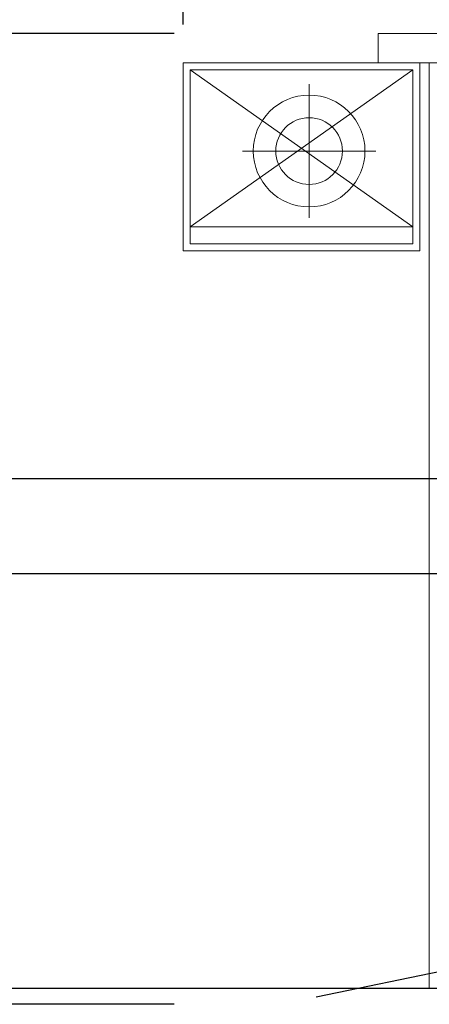
# Model space of a CAD drawing. Units: inches. Extents: x 2025 to 2528, y 1525 to 2336.
# Tile 11 of 18: x 2109 to 2138, y 2209 to 2278. Entities that reach past the tile are written whole.
import ezdxf

# ---------------------------------------------------------------- set-up
doc = ezdxf.new("R2010")
doc.units = ezdxf.units.IN
doc.layers.add('A-ANNO-DIMS', color=2, linetype='Continuous', lineweight=18)
doc.layers.add('A-FURN', color=8, linetype='Continuous', lineweight=18)
doc.styles.get("Standard").update_dxf_attribs({"font": 'arial.ttf'})
doc.dimstyles.new('Copy of ISO-25', dxfattribs={"dimtxt": 2.5, "dimasz": 2.5, "dimexe": 1.25, "dimexo": 0.625, "dimtad": 1, "dimdec": 1, "dimlunit": 4, "dimtxsty": 'Standard', "dimcen": 2.5, "dimadec": 0, "dimazin": 0, "dimtfac": 1, "dimtdec": 1, "dimtmove": 0, "dimatfit": 3, "dimfxl": 1, "dimarcsym": 0})

# ---------------------------------------------------------------- blocks, each defined once
blk = doc.blocks.new('*D6')
at = {"layer": 'A-ANNO-DIMS', "color": 0, "lineweight": -2, "transparency": 16777216}
for p, q in [((2075.013, 2282.787), (2075.013, 2237.927)), ((2255.013, 2282.787), (2255.013, 2237.927)), ((2077.513, 2239.177), (2252.513, 2239.177))]:
    blk.add_line(p, q, dxfattribs=at)
at = {"layer": 'A-ANNO-DIMS', "color": 0, "transparency": 16777216}
for points in [[(2077.513, 2239.594), (2077.513, 2238.761), (2075.013, 2239.177)], [(2252.513, 2239.594), (2252.513, 2238.761), (2255.013, 2239.177)]]:
    blk.add_solid(points, dxfattribs=at)
at = {"layer": 'Defpoints', "color": 0, "transparency": 16777216}
for p in [(2075.013, 2283.412), (2255.013, 2283.412), (2255.013, 2239.177)]:
    blk.add_point(p, dxfattribs=at)
at = {"layer": 'A-ANNO-DIMS', "color": 0, "transparency": 16777216, "insert": (2165.013, 2241.079), "char_height": 2.5, "attachment_point": 5}
blk.add_mtext("15'", dxfattribs=at)
blk = doc.blocks.new('A$C029D5C69')
for p, q in [((0.4164, 2.0693), (0.4164, 2.0066)), ((2.2315, 2.0693), (0.4164, 2.0693)), ((0, 1.606), (0, 2.0066)), ((0, 2.0066), (0.505, 2.0066)), ((0.4164, 2.0066), (2.2315, 2.0066)), ((0.505, 2.0066), (0.505, 1.606)), ((0.5252, 0.0351), (0.5252, 2.0066)), ((0.0151, 1.6211), (0.0151, 1.9915)), ((0.0151, 1.9915), (0.4899, 1.9915)), ((0.4899, 1.9915), (0.4899, 1.6211)), ((0.2689, 1.9609), (0.2689, 1.6764)), ((0.1267, 1.8186), (0.4111, 1.8186)), ((0.4899, 1.6211), (0.0151, 1.6211)), ((0.505, 1.606), (0, 1.606))]:
    blk.add_line(p, q)
at = {"ltscale": 0.005}
for p, q in [((0.4899, 1.6568), (0.0151, 1.9915)), ((0.0151, 1.6568), (0.4899, 1.9915)), ((0.0151, 1.6568), (0.4899, 1.6568))]:
    blk.add_line(p, q, dxfattribs=at)
for radius in [0.1191, 0.0711]:
    blk.add_circle((0.2689, 1.8186), radius)
blk = doc.blocks.new('*D56')
at = {"layer": 'A-ANNO-DIMS', "color": 0, "lineweight": -2, "transparency": 16777216}
for p, q in [((2120.208, 2277.944), (2120.208, 2291.728)), ((2207.933, 2277.944), (2207.933, 2291.728)), ((2122.708, 2290.478), (2205.433, 2290.478))]:
    blk.add_line(p, q, dxfattribs=at)
at = {"layer": 'A-ANNO-DIMS', "color": 0, "transparency": 16777216}
for points in [[(2122.708, 2290.895), (2122.708, 2290.061), (2120.208, 2290.478)], [(2205.433, 2290.895), (2205.433, 2290.061), (2207.933, 2290.478)]]:
    blk.add_solid(points, dxfattribs=at)
at = {"layer": 'Defpoints', "color": 0, "transparency": 16777216}
for p in [(2207.933, 2290.478), (2120.208, 2277.319), (2207.933, 2277.319)]:
    blk.add_point(p, dxfattribs=at)
at = {"layer": 'A-ANNO-DIMS', "color": 0, "transparency": 16777216, "insert": (2164.07, 2292.403), "char_height": 2.5, "attachment_point": 5}
blk.add_mtext('BED & NIGHTSTANDS 7\'-3 1/2" TYP.', dxfattribs=at)
blk = doc.blocks.new('*D57')
at = {"layer": 'A-ANNO-DIMS', "color": 0, "lineweight": -2, "transparency": 16777216}
for p, q in [((2119.583, 2277.319), (2105.799, 2277.319)), ((2107.049, 2211.264), (2107.049, 2274.819)), ((2119.583, 2208.764), (2105.799, 2208.764))]:
    blk.add_line(p, q, dxfattribs=at)
at = {"layer": 'A-ANNO-DIMS', "color": 0, "transparency": 16777216}
for points in [[(2106.632, 2274.819), (2107.466, 2274.819), (2107.049, 2277.319)], [(2106.632, 2211.264), (2107.466, 2211.264), (2107.049, 2208.764)]]:
    blk.add_solid(points, dxfattribs=at)
at = {"layer": 'Defpoints', "color": 0, "transparency": 16777216}
for p in [(2107.049, 2277.319), (2120.208, 2277.319), (2120.208, 2208.764)]:
    blk.add_point(p, dxfattribs=at)
at = {"layer": 'A-ANNO-DIMS', "color": 0, "transparency": 16777216, "insert": (2105.131, 2243.042), "char_height": 2.5, "attachment_point": 5, "rotation": 90}
blk.add_mtext('5\'-8 1/2" TYP.', dxfattribs=at)
blk = doc.blocks.new('*D78')
at = {"layer": 'A-ANNO-DIMS', "color": 0, "lineweight": -2, "transparency": 16777216}
for p, q in [((2254.388, 2245.877), (2027.213, 2245.877)), ((2028.463, 2212.377), (2028.463, 2243.377)), ((2254.388, 2209.877), (2027.213, 2209.877))]:
    blk.add_line(p, q, dxfattribs=at)
at = {"layer": 'A-ANNO-DIMS', "color": 0, "transparency": 16777216}
for points in [[(2028.046, 2243.377), (2028.88, 2243.377), (2028.463, 2245.877)], [(2028.046, 2212.377), (2028.88, 2212.377), (2028.463, 2209.877)]]:
    blk.add_solid(points, dxfattribs=at)
at = {"layer": 'Defpoints', "color": 0, "transparency": 16777216}
for p in [(2028.463, 2245.877), (2255.013, 2245.877), (2255.013, 2209.877)]:
    blk.add_point(p, dxfattribs=at)
at = {"layer": 'A-ANNO-DIMS', "color": 0, "transparency": 16777216, "insert": (2026.561, 2227.877), "char_height": 2.5, "attachment_point": 5, "rotation": 90}
blk.add_mtext('3\'-0"', dxfattribs=at)
blk = doc.blocks.new('*D80')
at = {"layer": 'A-ANNO-DIMS', "color": 0, "lineweight": -2, "transparency": 16777216}
for p, q in [((2065.388, 2292.412), (2027.213, 2292.412)), ((2028.463, 1566.912), (2028.463, 2289.912)), ((2285.388, 1564.412), (2027.213, 1564.412))]:
    blk.add_line(p, q, dxfattribs=at)
at = {"layer": 'A-ANNO-DIMS', "color": 0, "transparency": 16777216}
for points in [[(2028.046, 2289.912), (2028.88, 2289.912), (2028.463, 2292.412)], [(2028.046, 1566.912), (2028.88, 1566.912), (2028.463, 1564.412)]]:
    blk.add_solid(points, dxfattribs=at)
at = {"layer": 'Defpoints', "color": 0, "transparency": 16777216}
for p in [(2028.463, 2292.412), (2066.013, 2292.412), (2286.013, 1564.412)]:
    blk.add_point(p, dxfattribs=at)
at = {"layer": 'A-ANNO-DIMS', "color": 0, "transparency": 16777216, "insert": (2026.561, 1928.412), "char_height": 2.5, "attachment_point": 5, "rotation": 90}
blk.add_mtext('60\'-8"', dxfattribs=at)
blk = doc.blocks.new('*D81')
at = {"layer": 'A-ANNO-DIMS', "color": 0, "lineweight": -2, "transparency": 16777216}
for p, q in [((2175.825, 2218.922), (2152.347, 2214.024)), ((2129.625, 2209.285), (2149.9, 2213.514))]:
    blk.add_line(p, q, dxfattribs=at)
at = {"layer": 'A-ANNO-DIMS', "color": 0, "transparency": 16777216}
blk.add_solid([(2152.262, 2214.432), (2152.432, 2213.617), (2149.9, 2213.514)], dxfattribs=at)
at = {"layer": 'Defpoints', "color": 0, "transparency": 16777216}
for p in [(2149.9, 2213.514), (2129.625, 2209.285)]:
    blk.add_point(p, dxfattribs=at)
at = {"layer": 'A-ANNO-DIMS', "color": 0, "transparency": 16777216, "insert": (2164.918, 2218.607), "char_height": 2.5, "attachment_point": 5, "rotation": 11.7828}
blk.add_mtext('3X R1\'-8 1/2"', dxfattribs=at)

msp = doc.modelspace()

# ---------------------------------------------------------------- block references
at = {"layer": 'A-FURN', "xscale": 33.13032201413296, "yscale": 33.13032201413296, "zscale": 33.13032201413296}
msp.add_blockref('A$C029D5C69', (2120.208, 2208.764), dxfattribs=at)

# ---------------------------------------------------------------- dimensions: what is measured, and where the dimension line sits
at = {"layer": 'A-ANNO-DIMS'}
dim = msp.add_linear_dim(base=(2207.933, 2290.478), p1=(2120.208, 2277.319), p2=(2207.933, 2277.319), text='BED & NIGHTSTANDS <> TYP.', dimstyle='Copy of ISO-25', override={"dimdec": 1, "dimlfac": 1, "dimrnd": 0, "dimzin": 1, "dimdsep": 46, "dimlunit": 4, "dimfrac": 2}, dxfattribs=at)
dim.commit()
dim.dimension.update_dxf_attribs({"geometry": '*D56', "text_midpoint": (2164.07, 2292.403)})
for base, p1, p2, picture, middle in [((2028.463, 2292.412), (2286.013, 1564.412), (2066.013, 2292.412), '*D80', (2026.561, 1928.412)), ((2028.463, 2245.877), (2255.013, 2209.877), (2255.013, 2245.877), '*D78', (2026.561, 2227.877))]:
    dim = msp.add_linear_dim(base=base, p1=p1, p2=p2, angle=90, dimstyle='Copy of ISO-25', override={"dimdec": 1, "dimlfac": 1, "dimrnd": 0, "dimzin": 1, "dimdsep": 46, "dimlunit": 4, "dimfrac": 2}, dxfattribs=at)
    dim.commit()
    dim.dimension.update_dxf_attribs({"geometry": picture, "text_midpoint": middle})
dim = msp.add_linear_dim(base=(2255.013, 2239.177), p1=(2075.013, 2283.412), p2=(2255.013, 2283.412), dimstyle='Copy of ISO-25', override={"dimclrd": 0, "dimclre": 0, "dimclrt": 0}, dxfattribs=at)
dim.commit()
dim.dimension.update_dxf_attribs({"geometry": '*D6', "text_midpoint": (2165.013, 2241.079)})
dim = msp.add_linear_dim(base=(2107.049, 2277.319), p1=(2120.208, 2208.764), p2=(2120.208, 2277.319), angle=90, text='<> TYP.', dimstyle='Copy of ISO-25', override={"dimdec": 1, "dimlfac": 1, "dimrnd": 0, "dimzin": 1, "dimdsep": 46, "dimlunit": 4, "dimfrac": 2}, dxfattribs=at)
dim.commit()
dim.dimension.update_dxf_attribs({"geometry": '*D57', "text_midpoint": (2105.131, 2243.042)})
dim = msp.add_radius_dim(center=(2129.625, 2209.285), mpoint=(2149.9, 2213.514), text='3X <>', dimstyle='Copy of ISO-25', override={"dimdec": 1, "dimlfac": 1, "dimrnd": 0, "dimzin": 1, "dimdsep": 46, "dimlunit": 4, "dimfrac": 2}, dxfattribs=at)
dim.commit()
dim.dimension.update_dxf_attribs({"geometry": '*D81', "text_midpoint": (2164.918, 2218.607)})

doc.saveas('drawing.dxf')
